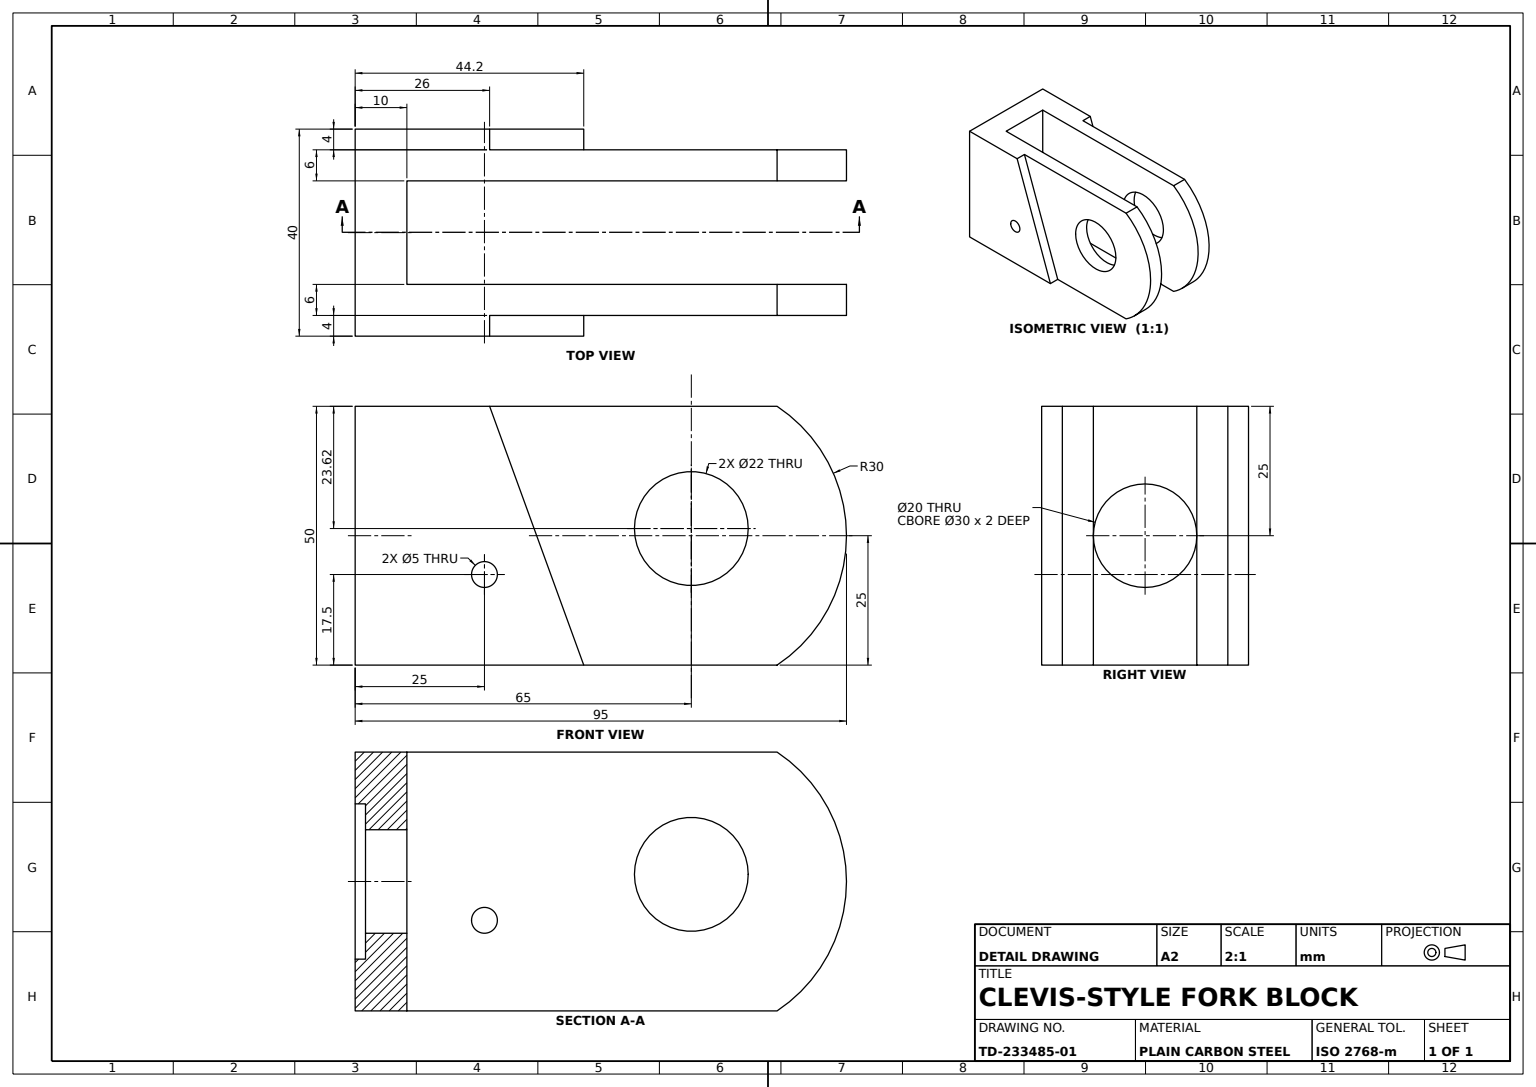
from build123d import *

# Parameters (mm, degrees)
SIDE_PLATE_DEPTH           = 10
MOUNTING_BLOCK_SKETCH_W    = 30
MOUNTING_BLOCK_SKETCH_H    = 50
MOUNTING_BLOCK_DEPTH       = 10
SECOND_START               = -10
SECOND_SIDE_PLATE_DEPTH    = 10
TOP_START                  = -4
TOP_RECESS_4MM_DEPTH       = 4
SIDE_RECESS_4MM_DEPTH      = 4
CROSS_HOLE_SKETCH_R        = 11
CROSS_HOLE_DEPTH           = 40
SPOT_FACE_SKETCH_R         = 15
SPOT_FACE_2MM_DEPTH        = 2
SMALL_HOLE_SKETCH_R        = 10
SMALL_HOLE_15MM_DEEP_DEPTH = 15
PIN_HOLE_SKETCH_R          = 2.5
PIN_HOLE_DEPTH             = 40


with BuildPart() as part:
    # Side Plate Sketch → Side Plate (new body)
    with BuildSketch(Plane.XY):
        with BuildLine():
            Line((0, 0), (0, -50))
            Line((0, -50), (61.578947368, -50))
            Line((61.578947368, -50), (77.289275323, -50))
            Line((77.289275323, -50), (81.583123952, -50))
            ThreePointArc((81.583123952, -50), (95, -25), (81.583123952, 0))
            Line((81.583123952, 0), (77.289275323, 0))
            Line((77.289275323, 0), (61.578947368, 0))
            Line((61.578947368, 0), (0, 0))
        make_face()
    extrude(amount=SIDE_PLATE_DEPTH)

    # Mounting Block Sketch → Mounting Block (add)
    with BuildSketch(Plane.ZY):
        with Locations((25, -25)):
            Rectangle(MOUNTING_BLOCK_SKETCH_W, MOUNTING_BLOCK_SKETCH_H)
    extrude(amount=-MOUNTING_BLOCK_DEPTH)

    # Second Plate Sketch → Second Side Plate (add)
    with BuildSketch(Plane.XY.offset(40).offset(SECOND_START)):
        with BuildLine():
            Line((10, 0), (81.583123952, 0))
            ThreePointArc((81.583123952, 0), (95, -25), (81.583123952, -50))
            Line((81.583123952, -50), (10, -50))
            Line((10, -50), (10, 0))
        make_face()
    extrude(amount=SECOND_SIDE_PLATE_DEPTH)

    # Top Recess Sketch → Top Recess 4mm (cut)
    with BuildSketch(Plane.XY.offset(40).offset(TOP_START)):
        with BuildLine():
            Line((81.583123952, 0), (26, 0))
            Line((26, 0), (44.196790465, -50))
            Line((44.196790465, -50), (81.583123952, -50))
            ThreePointArc((81.583123952, -50), (95, -25), (81.583123952, 0))
        make_face()
    extrude(amount=TOP_RECESS_4MM_DEPTH, mode=Mode.SUBTRACT)

    # Side Recess Sketch → Side Recess 4mm (cut)
    with BuildSketch(Plane(origin=(0, 0, 0), x_dir=(-1, 0, 0), z_dir=(0, 0, -1))):
        with BuildLine():
            Line((-26, 0), (-44.2, -50))
            Line((-44.2, -50), (-81.583123952, -50))
            ThreePointArc((-81.583123952, -50), (-95, -25), (-81.583123952, 0))
            Line((-81.583123952, 0), (-26, 0))
        make_face()
    extrude(amount=-SIDE_RECESS_4MM_DEPTH, mode=Mode.SUBTRACT)

    # Cross Hole Sketch → Cross Hole (cut)
    with BuildSketch(Plane.XY.offset(36)):
        with Locations((65, -23.619190871)):
            Circle(CROSS_HOLE_SKETCH_R)
    extrude(amount=-CROSS_HOLE_DEPTH, mode=Mode.SUBTRACT)

    # Spot Face Sketch → Spot Face 2mm (cut)
    with BuildSketch(Plane.ZY):
        with Locations(Location((20, -25, 0), (0, 0, 270))):
            Circle(SPOT_FACE_SKETCH_R)
    extrude(amount=-SPOT_FACE_2MM_DEPTH, mode=Mode.SUBTRACT)

    # Small Hole Sketch → Small Hole 15mm Deep (cut)
    with BuildSketch(Plane.ZY.offset(-2)):
        with Locations(Location((20, -25, 0), (0, 0, 270))):
            Circle(SMALL_HOLE_SKETCH_R)
    extrude(amount=-SMALL_HOLE_15MM_DEEP_DEPTH, mode=Mode.SUBTRACT)

    # Pin Hole Sketch → Pin Hole (cut)
    with BuildSketch(Plane.XY.offset(40)):
        with Locations((25, -32.5)):
            Circle(PIN_HOLE_SKETCH_R)
    extrude(amount=-PIN_HOLE_DEPTH, mode=Mode.SUBTRACT)


solid = part.part
